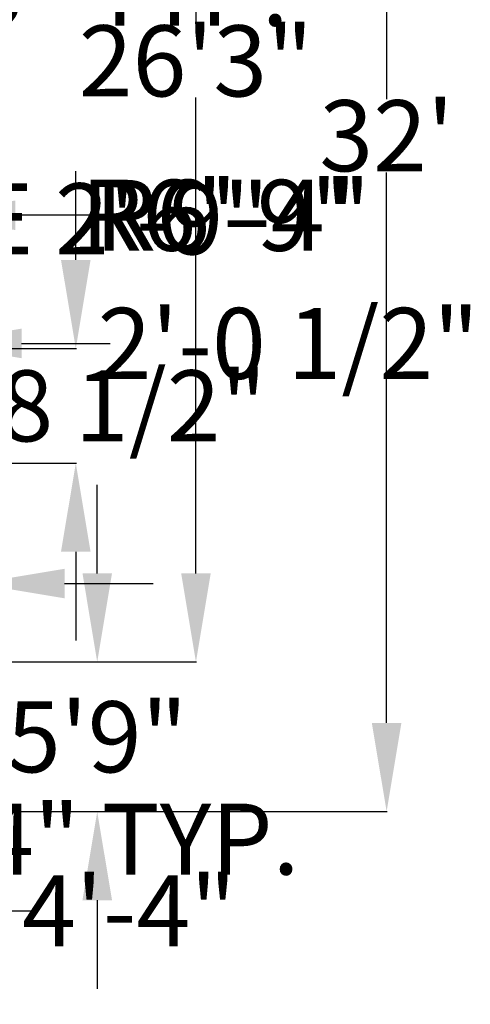
# Model space of a CAD drawing. Units: inches. Extents: x 25 to 82118, y 10 to 6494.
# Tile 7 of 9: x 41087 to 41215, y 3093 to 3373. Entities that reach past the tile are written whole.
import ezdxf

# ---------------------------------------------------------------- set-up
doc = ezdxf.new("R2010")
doc.units = ezdxf.units.IN
doc.header["$MEASUREMENT"] = 0
doc.layers.add('A-ANNO-DIMS', color=2, linetype='Continuous', lineweight=18)
doc.styles.get("Standard").update_dxf_attribs({"font": 'arial.ttf'})
doc.dimstyles.get("Standard").update_dxf_attribs({"dimtxt": 20.18, "dimasz": 25.18, "dimexe": 0.18, "dimexo": 0.0625, "dimgap": 0.09, "dimtad": 0, "dimtih": 1, "dimtoh": 1, "dimdec": 0, "dimzin": 0, "dimdsep": 46, "dimlunit": 3, "dimtxsty": 'Standard', "dimcen": 0.09, "dimadec": 0, "dimazin": 0, "dimtfac": 1, "dimtdec": 0, "dimtofl": 0, "dimtmove": 0, "dimatfit": 3, "dimfxl": 1, "dimtolj": 1, "dimtzin": 0, "dimarcsym": 0})

# ---------------------------------------------------------------- blocks, each defined once
blk = doc.blocks.new('*D15')
at = {"layer": 'A-ANNO-DIMS', "color": 0, "lineweight": -2, "transparency": 16777216}
for p, q in [((41074.27, 3531.88), (41136.86, 3531.88)), ((41136.68, 3506.7), (41136.68, 3371.51)), ((41136.68, 3215.52), (41136.68, 3350.71)), ((41074.27, 3190.34), (41136.86, 3190.34))]:
    blk.add_line(p, q, dxfattribs=at)
at = {"layer": 'A-ANNO-DIMS', "color": 0, "transparency": 16777216}
for points in [[(41132.48, 3506.7), (41140.87, 3506.7), (41136.68, 3531.88)], [(41132.48, 3215.52), (41140.87, 3215.52), (41136.68, 3190.34)]]:
    blk.add_solid(points, dxfattribs=at)
at = {"layer": 'Defpoints', "color": 0, "transparency": 16777216}
for p in [(41074.21, 3531.88), (41074.21, 3190.34), (41136.68, 3190.34)]:
    blk.add_point(p, dxfattribs=at)
at = {"layer": 'A-ANNO-DIMS', "color": 0, "transparency": 16777216, "insert": (41136.68, 3361.11), "char_height": 20.18, "attachment_point": 5}
blk.add_mtext('\\A1;26\'3"', dxfattribs=at)
blk = doc.blocks.new('*D16')
at = {"layer": 'A-ANNO-DIMS', "color": 0, "lineweight": -2, "transparency": 16777216}
for p, q in [((41074.33, 3531.88), (41191.01, 3531.88)), ((41190.83, 3506.7), (41190.83, 3350.25)), ((41190.83, 3173), (41190.83, 3329.45)), ((41074.33, 3147.82), (41191.01, 3147.82))]:
    blk.add_line(p, q, dxfattribs=at)
at = {"layer": 'A-ANNO-DIMS', "color": 0, "transparency": 16777216}
for points in [[(41186.63, 3506.7), (41195.02, 3506.7), (41190.83, 3531.88)], [(41186.63, 3173), (41195.02, 3173), (41190.83, 3147.82)]]:
    blk.add_solid(points, dxfattribs=at)
at = {"layer": 'Defpoints', "color": 0, "transparency": 16777216}
for p in [(41074.27, 3531.88), (41074.27, 3147.82), (41190.83, 3147.82)]:
    blk.add_point(p, dxfattribs=at)
at = {"layer": 'A-ANNO-DIMS', "color": 0, "transparency": 16777216, "insert": (41190.83, 3339.85), "char_height": 20.18, "attachment_point": 5}
blk.add_mtext("\\A1;32'", dxfattribs=at)
blk = doc.blocks.new('*D17')
at = {"layer": 'A-ANNO-DIMS', "color": 0, "lineweight": -2, "transparency": 16777216}
for p, q in [((41108.65, 3215.52), (41108.65, 3240.7)), ((41074.27, 3190.34), (41108.83, 3190.34)), ((41074.4, 3147.82), (41108.83, 3147.82)), ((41108.65, 3122.64), (41108.65, 3097.46))]:
    blk.add_line(p, q, dxfattribs=at)
at = {"layer": 'A-ANNO-DIMS', "color": 0, "transparency": 16777216}
for points in [[(41104.46, 3215.52), (41112.85, 3215.52), (41108.65, 3190.34)], [(41104.46, 3122.64), (41112.85, 3122.64), (41108.65, 3147.82)]]:
    blk.add_solid(points, dxfattribs=at)
at = {"layer": 'Defpoints', "color": 0, "transparency": 16777216}
for p in [(41074.21, 3190.34), (41074.33, 3147.82), (41108.65, 3147.82)]:
    blk.add_point(p, dxfattribs=at)
at = {"layer": 'A-ANNO-DIMS', "color": 0, "transparency": 16777216, "insert": (41108.65, 3169.08), "char_height": 20.18, "attachment_point": 5}
blk.add_mtext('\\A1;5\'9"', dxfattribs=at)
blk = doc.blocks.new('*D27')
at = {"layer": 'A-ANNO-DIMS', "color": 0, "lineweight": -2, "transparency": 16777216}
for p, q in [((40878.03, 3381.2), (40852.85, 3381.2)), ((40903.21, 3382.03), (40903.21, 3381.02)), ((40909.21, 3382.03), (40909.21, 3381.02)), ((40934.39, 3381.2), (40959.57, 3381.2))]:
    blk.add_line(p, q, dxfattribs=at)
at = {"layer": 'A-ANNO-DIMS', "color": 0, "transparency": 16777216}
for points in [[(40878.03, 3385.39), (40878.03, 3377), (40903.21, 3381.2)], [(40934.39, 3385.39), (40934.39, 3377), (40909.21, 3381.2)]]:
    blk.add_solid(points, dxfattribs=at)
at = {"layer": 'Defpoints', "color": 0, "transparency": 16777216}
for p in [(40903.21, 3382.1), (40909.21, 3382.1), (40909.21, 3381.2)]:
    blk.add_point(p, dxfattribs=at)
at = {"layer": 'A-ANNO-DIMS', "color": 0, "transparency": 16777216, "insert": (41062.95, 3381.2), "char_height": 20.18, "attachment_point": 5}
blk.add_mtext('\\A1;POST 0\'-6" TYP.', dxfattribs=at)
blk = doc.blocks.new('*D31')
at = {"layer": 'A-ANNO-DIMS', "color": 0, "lineweight": -2, "transparency": 16777216}
for p, q in [((40838.63, 3147.76), (40838.63, 3139.84)), ((40890.63, 3147.76), (40890.63, 3139.84)), ((40863.81, 3140.02), (40865.45, 3140.02)), ((40890.63, 3140.02), (40915.81, 3140.02))]:
    blk.add_line(p, q, dxfattribs=at)
at = {"layer": 'A-ANNO-DIMS', "color": 0, "transparency": 16777216}
for points in [[(40863.81, 3144.22), (40863.81, 3135.82), (40838.63, 3140.02)], [(40865.45, 3144.22), (40865.45, 3135.82), (40890.63, 3140.02)]]:
    blk.add_solid(points, dxfattribs=at)
at = {"layer": 'Defpoints', "color": 0, "transparency": 16777216}
for p in [(40838.63, 3147.82), (40890.63, 3147.82), (40890.63, 3140.02)]:
    blk.add_point(p, dxfattribs=at)
at = {"layer": 'A-ANNO-DIMS', "color": 0, "transparency": 16777216, "insert": (41043.59, 3140.02), "char_height": 20.18, "attachment_point": 5}
blk.add_mtext('\\A1;WINDOW 4\'-4" TYP.', dxfattribs=at)
blk = doc.blocks.new('*D43')
at = {"layer": 'A-ANNO-DIMS', "color": 0, "lineweight": -2, "transparency": 16777216}
for p, q in [((41029.25, 3357.91), (41029.25, 3383.09)), ((41024.37, 3332.73), (41029.43, 3332.73)), ((41024.37, 3299.75), (41029.43, 3299.75)), ((41029.25, 3274.57), (41029.25, 3249.39))]:
    blk.add_line(p, q, dxfattribs=at)
at = {"layer": 'A-ANNO-DIMS', "color": 0, "transparency": 16777216}
for points in [[(41025.05, 3357.91), (41033.45, 3357.91), (41029.25, 3332.73)], [(41025.05, 3274.57), (41033.45, 3274.57), (41029.25, 3299.75)]]:
    blk.add_solid(points, dxfattribs=at)
at = {"layer": 'Defpoints', "color": 0, "transparency": 16777216}
for p in [(41024.3, 3332.73), (41029.25, 3332.73), (41024.3, 3299.75)]:
    blk.add_point(p, dxfattribs=at)
at = {"layer": 'A-ANNO-DIMS', "color": 0, "transparency": 16777216, "insert": (41029.25, 3316.24), "char_height": 20.18, "attachment_point": 5}
blk.add_mtext('\\A1;COFFEE TABLE 2\'-9"', dxfattribs=at)
blk = doc.blocks.new('*D46')
at = {"layer": 'A-ANNO-DIMS', "color": 0, "lineweight": -2, "transparency": 16777216}
for p, q in [((41037.52, 3289.18), (41037.52, 3280.66)), ((41061.97, 3289.18), (41061.97, 3280.66)), ((41012.34, 3280.84), (40987.16, 3280.84)), ((41087.15, 3280.84), (41112.33, 3280.84))]:
    blk.add_line(p, q, dxfattribs=at)
at = {"layer": 'A-ANNO-DIMS', "color": 0, "transparency": 16777216}
for points in [[(41012.34, 3285.04), (41012.34, 3276.64), (41037.52, 3280.84)], [(41087.15, 3285.04), (41087.15, 3276.64), (41061.97, 3280.84)]]:
    blk.add_solid(points, dxfattribs=at)
at = {"layer": 'Defpoints', "color": 0, "transparency": 16777216}
for p in [(41037.52, 3289.24), (41061.97, 3289.24), (41061.97, 3280.84)]:
    blk.add_point(p, dxfattribs=at)
at = {"layer": 'A-ANNO-DIMS', "color": 0, "transparency": 16777216, "insert": (41162.92, 3280.84), "char_height": 20.18, "attachment_point": 5}
blk.add_mtext('\\A1;2\'-0 1/2"', dxfattribs=at)
blk = doc.blocks.new('*D65')
at = {"layer": 'A-ANNO-DIMS', "color": 0, "lineweight": -2, "transparency": 16777216}
for p, q in [((41102.56, 3304.59), (41102.56, 3329.77)), ((41065.27, 3279.41), (41102.74, 3279.41)), ((41065.27, 3246.82), (41102.74, 3246.82)), ((41102.56, 3221.64), (41102.56, 3196.46))]:
    blk.add_line(p, q, dxfattribs=at)
at = {"layer": 'A-ANNO-DIMS', "color": 0, "transparency": 16777216}
for points in [[(41098.36, 3304.59), (41106.76, 3304.59), (41102.56, 3279.41)], [(41098.36, 3221.64), (41106.76, 3221.64), (41102.56, 3246.82)]]:
    blk.add_solid(points, dxfattribs=at)
at = {"layer": 'Defpoints', "color": 0, "transparency": 16777216}
for p in [(41065.21, 3279.41), (41102.56, 3279.41), (41065.21, 3246.82)]:
    blk.add_point(p, dxfattribs=at)
at = {"layer": 'A-ANNO-DIMS', "color": 0, "transparency": 16777216, "insert": (41102.56, 3263.11), "char_height": 20.18, "attachment_point": 5}
blk.add_mtext('\\A1;2\'-8 1/2"', dxfattribs=at)
blk = doc.blocks.new('*D66')
at = {"layer": 'A-ANNO-DIMS', "color": 0, "lineweight": -2, "transparency": 16777216}
for p, q in [((41013.21, 3522.76), (41013.21, 3119.41)), ((41065.21, 3522.76), (41065.21, 3119.41)), ((41038.39, 3119.59), (41040.03, 3119.59)), ((41065.21, 3119.59), (41090.39, 3119.59))]:
    blk.add_line(p, q, dxfattribs=at)
at = {"layer": 'A-ANNO-DIMS', "color": 0, "transparency": 16777216}
for points in [[(41038.39, 3123.78), (41038.39, 3115.39), (41013.21, 3119.59)], [(41040.03, 3123.78), (41040.03, 3115.39), (41065.21, 3119.59)]]:
    blk.add_solid(points, dxfattribs=at)
at = {"layer": 'Defpoints', "color": 0, "transparency": 16777216}
for p in [(41013.21, 3522.82), (41065.21, 3522.82), (41065.21, 3119.59)]:
    blk.add_point(p, dxfattribs=at)
at = {"layer": 'A-ANNO-DIMS', "color": 0, "transparency": 16777216, "insert": (41117.71, 3119.59), "char_height": 20.18, "attachment_point": 5}
blk.add_mtext('\\A1;4\'-4"', dxfattribs=at)
blk = doc.blocks.new('*D68')
at = {"layer": 'A-ANNO-DIMS', "color": 0, "lineweight": -2, "transparency": 16777216}
for p, q in [((41052.05, 3240.76), (41052.05, 3212.44)), ((41074.21, 3240.76), (41074.21, 3212.44)), ((41026.87, 3212.62), (41001.69, 3212.62)), ((41099.39, 3212.62), (41124.57, 3212.62))]:
    blk.add_line(p, q, dxfattribs=at)
at = {"layer": 'A-ANNO-DIMS', "color": 0, "transparency": 16777216}
for points in [[(41026.87, 3216.82), (41026.87, 3208.42), (41052.05, 3212.62)], [(41099.39, 3216.82), (41099.39, 3208.42), (41074.21, 3212.62)]]:
    blk.add_solid(points, dxfattribs=at)
at = {"layer": 'Defpoints', "color": 0, "transparency": 16777216}
for p in [(41052.05, 3240.82), (41074.21, 3240.82), (41052.05, 3212.62)]:
    blk.add_point(p, dxfattribs=at)
at = {"layer": 'A-ANNO-DIMS', "color": 0, "transparency": 16777216, "insert": (40967.89, 3212.62), "char_height": 20.18, "attachment_point": 5}
blk.add_mtext('\\A1;1\'-10"', dxfattribs=at)
blk = doc.blocks.new('*D69')
at = {"layer": 'A-ANNO-DIMS', "color": 0, "lineweight": -2, "transparency": 16777216}
for p, q in [((40975.29, 3317.24), (40975.47, 3317.24)), ((40975.38, 3317.15), (40975.38, 3317.33)), ((41106.55, 3317.24), (41081.37, 3317.24))]:
    blk.add_line(p, q, dxfattribs=at)
at = {"layer": 'A-ANNO-DIMS', "color": 0, "transparency": 16777216}
blk.add_solid([(41081.37, 3321.44), (41081.37, 3313.05), (41056.19, 3317.24)], dxfattribs=at)
at = {"layer": 'Defpoints', "color": 0, "transparency": 16777216}
for p in [(40975.38, 3317.24), (41056.19, 3317.24)]:
    blk.add_point(p, dxfattribs=at)
at = {"layer": 'A-ANNO-DIMS', "color": 0, "transparency": 16777216, "insert": (41143.12, 3317.24), "char_height": 20.18, "attachment_point": 5}
blk.add_mtext('\\A1;R6\'-9"', dxfattribs=at)
blk = doc.blocks.new('*D70')
at = {"layer": 'A-ANNO-DIMS', "color": 0, "lineweight": -2, "transparency": 16777216}
for p, q in [((40983.92, 3317.24), (40984.1, 3317.24)), ((40984.01, 3317.15), (40984.01, 3317.33)), ((41110.55, 3317.24), (41085.37, 3317.24))]:
    blk.add_line(p, q, dxfattribs=at)
at = {"layer": 'A-ANNO-DIMS', "color": 0, "transparency": 16777216}
blk.add_solid([(41085.37, 3321.44), (41085.37, 3313.05), (41060.19, 3317.24)], dxfattribs=at)
at = {"layer": 'Defpoints', "color": 0, "transparency": 16777216}
for p in [(40984.01, 3317.24), (41060.19, 3317.24)]:
    blk.add_point(p, dxfattribs=at)
at = {"layer": 'A-ANNO-DIMS', "color": 0, "transparency": 16777216, "insert": (41147.12, 3317.24), "char_height": 20.18, "attachment_point": 5}
blk.add_mtext('\\A1;R6\'-4"', dxfattribs=at)

msp = doc.modelspace()

# ---------------------------------------------------------------- dimensions: what is measured, and where the dimension line sits
at = {"layer": 'A-ANNO-DIMS'}
for base, p1, p2, text, override, picture, middle in [((41136.68, 3190.34), (41074.21, 3531.88), (41074.21, 3190.34), '26\'3"', {"dimclrd": 0, "dimclre": 0, "dimclrt": 0}, '*D15', (41136.68, 3361.11)), ((41029.25, 3332.73), (41024.3, 3299.75), (41024.3, 3332.73), 'COFFEE TABLE <>', {"dimdec": 1, "dimlfac": 1, "dimrnd": 0, "dimzin": 1, "dimdsep": 46, "dimlunit": 4, "dimfrac": 2}, '*D43', (41029.25, 3316.24)), ((41108.65, 3147.82), (41074.21, 3190.34), (41074.33, 3147.82), '5\'9"', {"dimclrd": 0, "dimclre": 0, "dimclrt": 0}, '*D17', (41108.65, 3169.08))]:
    dim = msp.add_linear_dim(base=base, p1=p1, p2=p2, angle=90, text=text, dimstyle='Standard', override=override, dxfattribs=at)
    dim.commit()
    dim.dimension.update_dxf_attribs({"geometry": picture, "text_midpoint": middle})
for base, p1, p2, angle, override, picture, middle in [((41190.83, 3147.82), (41074.27, 3531.88), (41074.27, 3147.82), 90, {"dimclrd": 0, "dimclre": 0, "dimclrt": 0}, '*D16', (41190.83, 3339.85)), ((41102.56, 3279.41), (41065.21, 3246.82), (41065.21, 3279.41), 90, {"dimdec": 1, "dimlfac": 1, "dimrnd": 0, "dimzin": 1, "dimdsep": 46, "dimlunit": 4, "dimfrac": 2}, '*D65', (41102.56, 3263.11)), ((41052.05, 3212.62), (41074.21, 3240.82), (41052.05, 3240.82), 180, {"dimdec": 1, "dimlfac": 1, "dimrnd": 0, "dimzin": 1, "dimdsep": 46, "dimlunit": 4, "dimfrac": 2}, '*D68', (40967.89, 3212.62))]:
    dim = msp.add_linear_dim(base=base, p1=p1, p2=p2, angle=angle, dimstyle='Standard', override=override, dxfattribs=at)
    dim.commit()
    dim.dimension.update_dxf_attribs({"geometry": picture, "text_midpoint": middle})
for base, p1, p2, picture, middle in [((41065.21, 3119.59), (41013.21, 3522.82), (41065.21, 3522.82), '*D66', (41117.71, 3119.59)), ((41061.9692, 3280.8387), (41037.5212, 3289.2399), (41061.9692, 3289.2399), '*D46', (41162.9243, 3280.8387))]:
    dim = msp.add_linear_dim(base=base, p1=p1, p2=p2, dimstyle='Standard', override={"dimdec": 1, "dimlfac": 1, "dimrnd": 0, "dimzin": 1, "dimdsep": 46, "dimlunit": 4, "dimfrac": 2}, dxfattribs=at)
    dim.commit()
    dim.dimension.update_dxf_attribs({"geometry": picture, "text_midpoint": middle})
for base, p1, p2, text, picture, middle in [((40909.21, 3381.2), (40903.21, 3382.1), (40909.21, 3382.1), 'POST <> TYP.', '*D27', (41062.95, 3381.2)), ((40890.63, 3140.02), (40838.63, 3147.82), (40890.63, 3147.82), 'WINDOW <> TYP.', '*D31', (41043.59, 3140.02))]:
    dim = msp.add_linear_dim(base=base, p1=p1, p2=p2, text=text, dimstyle='Standard', override={"dimdec": 1, "dimlfac": 1, "dimrnd": 0, "dimzin": 1, "dimdsep": 46, "dimlunit": 4, "dimfrac": 2}, dxfattribs=at)
    dim.commit()
    dim.dimension.update_dxf_attribs({"geometry": picture, "text_midpoint": middle})
for center, mpoint, picture, middle in [((40975.38, 3317.24), (41056.19, 3317.24), '*D69', (41143.12, 3317.24)), ((40984.01, 3317.24), (41060.19, 3317.24), '*D70', (41147.12, 3317.24))]:
    dim = msp.add_radius_dim(center=center, mpoint=mpoint, dimstyle='Standard', override={"dimdec": 1, "dimlfac": 1, "dimrnd": 0, "dimzin": 1, "dimdsep": 46, "dimlunit": 4, "dimfrac": 2}, dxfattribs=at)
    dim.commit()
    dim.dimension.update_dxf_attribs({"geometry": picture, "text_midpoint": middle})

doc.saveas('drawing.dxf')
